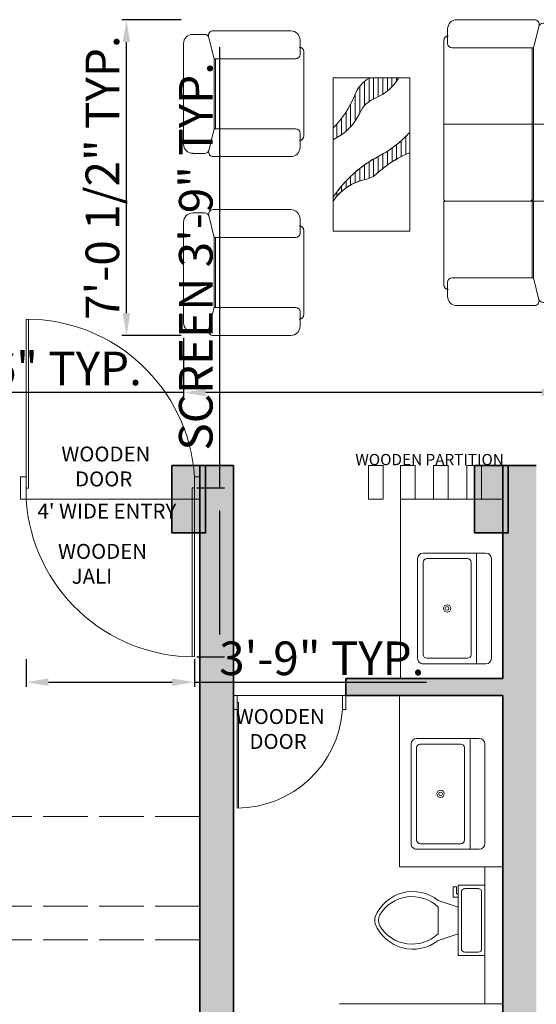
# Model space of a CAD drawing. Units: millimetres. Extents: x 595116 to 630915, y 909473 to 920225.
# Tile 130 of 134: x 630446 to 630585, y 919466 to 919729. Entities that reach past the tile are written whole.
import ezdxf

# ---------------------------------------------------------------- set-up
doc = ezdxf.new("R2010")
doc.units = ezdxf.units.MM
doc.linetypes.add('ACAD_ISO02W100', pattern=[15, 12, -3])
for name, color, linetype, lineweight in [('A-FLOR-FIXT', 9, 'Continuous', 18), ('A-FLOR-SCRN', 31, 'Continuous', 18), ('A-FLOR-SCRN-OVHD', 31, 'ACAD_ISO02W100', 13), ('A-FURN', 32, 'Continuous', 18), ('A-WALL', 1, 'Continuous', 35), ('A-WALL-PATT', 8, 'Continuous', 13), ('Column', 6, 'Continuous', 35), ('Dimension', 3, 'Continuous', 18), ('Doors', 31, 'Continuous', 20), ('Text', 7, 'Continuous', 18)]:
    doc.layers.add(name, color=color, linetype=linetype, lineweight=lineweight)
doc.styles.get("Standard").update_dxf_attribs({"font": 'arial.ttf'})
doc.dimstyles.new('ISO-25', dxfattribs={"dimtxt": 9, "dimasz": 6, "dimexe": 1.25, "dimexo": 0.625, "dimtad": 1, "dimlunit": 4, "dimtxsty": 'Standard', "dimcen": 2.5, "dimadec": 0, "dimazin": 0, "dimtfac": 1, "dimtmove": 0, "dimatfit": 3, "dimfxl": 1, "dimarcsym": 0})

# ---------------------------------------------------------------- blocks, each defined once
blk = doc.blocks.new('KWD')
for points in [[(629753.63, 919957.93), (629752.54, 919957.93), (629752.54, 919953.43), (629753.63, 919953.43)], [(629787.45, 919957.93), (629787.45, 919953.43), (629788.54, 919953.43), (629788.54, 919957.93)]]:
    blk.add_lwpolyline(points, close=True)
blk.add_lwpolyline([(629753.63, 919921.79), (629753.63, 919955.68), (629754.13, 919955.68), (629754.13, 919921.8)])
blk.add_arc((629753.64, 919955.68), 33.88, 269.99, 356.196)
blk = doc.blocks.new('DS')
blk.add_lwpolyline([(630069.78, 919993.92), (630069.78, 919965.68), (630069.37, 919965.68), (630069.37, 919993.91)])
for points in [[(630041.6, 919963.81), (630041.6, 919967.56), (630040.69, 919967.56), (630040.69, 919963.81)], [(630069.78, 919963.81), (630070.69, 919963.81), (630070.69, 919967.56), (630069.78, 919967.56)]]:
    blk.add_lwpolyline(points, close=True)
blk.add_arc((630069.78, 919965.69), 28.24, 89.99, 176.196)
blk = doc.blocks.new('Sink-single - 30 in top')
blk.add_line((-15, -3.999996), (15, -3.999996))
for points in [[(-13.5, 0), (13.5, 0)], [(-15, -18.499996), (-15, -1.5)], [(15, -1.5), (15, -18.499996)], [(-13.5, -17.499996), (-13.5, -6.499996)], [(-12.5, -5.499996), (12.5, -5.499996)], [(13.5, -6.499996), (13.5, -17.499996)], [(12.5, -18.499996), (-12.5, -18.499996)], [(13.5, -19.999996), (-13.5, -19.999996)]]:
    blk.add_lwpolyline(points)
for radius in [1, 0.5]:
    blk.add_circle((0, -11.999996), radius)
for centre, radius, start, end in [((-13.5, -1.5), 1.5, 90, 180), ((13.5, -1.5), 1.5, 0, 90), ((-12.5, -6.499996), 1, 90, 180), ((12.5, -6.499996), 1, 0, 90), ((-13.5, -18.499996), 1.5, 180, 270), ((-12.5, -17.499996), 1, 180, 270), ((12.5, -17.499996), 1, 270, 0), ((13.5, -18.499996), 1.5, 270, 0)]:
    blk.add_arc(centre, radius, start, end)
blk = doc.blocks.new('Toilet - top')
for p, q in [((9.5, -6), (9.5, -2)), ((-10, -8.5), (-8, -8.5)), ((-10, -9.5), (-10, -8.5)), ((-8, -8.5), (-8, -8)), ((-7, -8), (-7, -9.5)), ((-4, -8), (-6, -14)), ((4, -8), (6, -14)), ((-7, -9.5), (-10, -9.5)), ((4, -14), (-4, -14))]:
    blk.add_line(p, q)
blk.add_lwpolyline([(10.5, -8), (10.5, 0), (-10.5, 0), (-10.5, -8)], close=True)
for points in [[(-9.5, -2), (-9.5, -6)], [(8.5, -1), (-8.5, -1)], [(-8.5, -7), (8.5, -7)]]:
    blk.add_lwpolyline(points)
for centre, radius, start, end in [((-8.62, -1.88), 0.884, 81.8699, 188.1301), ((8.62, -1.88), 0.884, 351.8699, 98.1301), ((-8.62, -6.12), 0.884, 171.8699, 278.1301), ((8.62, -6.12), 0.884, 261.8699, 8.1301), ((3.52, -21.58), 12.17, 141.4691, 247.9714), ((4.2, -21.82), 11.33, 136.3677, 238.9468), ((-3.52, -21.58), 12.17, 292.0284, 38.5307), ((-4.2, -21.82), 11.33, 301.053, 43.6321), ((0, -27.88), 4, 245.7318, 294.2682), ((0, -29), 4, 254.8605, 285.1395)]:
    blk.add_arc(centre, radius, start, end)
blk = doc.blocks.new('SOFA')
for p, q in [((629520.59, 919742.63), (629517.45, 919742.63)), ((629517.45, 919742.63), (629520.59, 919742.63)), ((629543.7, 919743.59), (629522.89, 919743.59)), ((629522.89, 919743.59), (629543.7, 919743.59)), ((629514.98, 919740.17), (629514.98, 919695.65)), ((629514.98, 919695.65), (629514.98, 919740.17)), ((629521.79, 919741.7), (629521.7, 919742.06)), ((629521.7, 919742.06), (629523.2, 919736.06)), ((629546.16, 919741.12), (629546.16, 919739.22)), ((629546.16, 919741.12), (629546.16, 919737.29)), ((629588.11, 919740.62), (629608.91, 919740.62)), ((629588.11, 919740.62), (629608.91, 919740.62)), ((629547.17, 919738.01), (629547.17, 919695.65)), ((629547.17, 919738.01), (629547.17, 919695.65)), ((629585.64, 919738.15), (629585.64, 919734.33)), ((629585.64, 919736.25), (629585.64, 919738.15)), ((629610.11, 919739.09), (629608.61, 919733.09)), ((629610.11, 919739.09), (629610.02, 919738.73)), ((629611.21, 919739.66), (629614.36, 919739.66)), ((629611.21, 919739.66), (629614.36, 919739.66)), ((629523.2, 919736.06), (629523.2, 919695.65)), ((629523.2, 919695.65), (629523.2, 919736.06)), ((629523.2, 919695.65), (629523.2, 919736.06)), ((629544.93, 919736.06), (629523.2, 919736.06)), ((629523.2, 919736.06), (629523.53, 919736.06)), ((629523.2, 919736.06), (629523.53, 919736.06)), ((629523.53, 919736.06), (629523.53, 919695.65)), ((629523.53, 919736.06), (629523.53, 919695.65)), ((629523.53, 919736.06), (629523.53, 919695.65)), ((629584.64, 919735.04), (629584.64, 919712.53)), ((629584.64, 919712.53), (629584.64, 919735.04)), ((629616.82, 919737.2), (629616.82, 919710.3)), ((629616.82, 919737.2), (629616.82, 919710.3)), ((629586.87, 919733.09), (629608.61, 919733.09)), ((629608.28, 919733.09), (629608.61, 919733.09)), ((629608.28, 919714.4), (629608.28, 919733.09)), ((629608.28, 919733.09), (629608.28, 919714.4)), ((629608.61, 919733.09), (629608.61, 919714.4)), ((629608.61, 919733.09), (629608.61, 919714.4)), ((629556.25, 919728.06), (629556.25, 919687.01)), ((629556.25, 919687.01), (629556.25, 919728.06)), ((629576.77, 919728.06), (629556.25, 919728.06)), ((629556.25, 919728.06), (629576.77, 919728.06)), ((629559.82, 919728), (629559.82, 919727.13)), ((629561.06, 919728), (629561.06, 919725.63)), ((629562.29, 919728), (629562.29, 919724.5)), ((629563.52, 919728), (629563.52, 919723.63)), ((629564.75, 919728), (629564.75, 919722.96)), ((629565.98, 919728), (629565.98, 919722.42)), ((629567.19, 919727.97), (629567.19, 919721.68)), ((629568.42, 919727.08), (629568.42, 919720.54)), ((629576.77, 919687.01), (629576.77, 919728.06)), ((629576.77, 919728.06), (629576.77, 919687.01)), ((629569.65, 919725.8), (629569.65, 919718.67)), ((629569.65, 919725.8), (629569.65, 919718.67)), ((629570.88, 919723.75), (629570.88, 919716.49)), ((629570.88, 919716.49), (629570.88, 919723.75)), ((629572.12, 919720.99), (629572.12, 919714.94)), ((629573.35, 919718.86), (629573.35, 919713.74)), ((629574.58, 919717.12), (629574.58, 919712.78)), ((629547.17, 919715.59), (629514.98, 919715.59)), ((629575.81, 919715.64), (629575.81, 919712.02)), ((629586.87, 919714.4), (629608.61, 919714.4)), ((629608.61, 919714.4), (629608.28, 919714.4)), ((629610.09, 919708.48), (629608.61, 919714.4)), ((629557.33, 919712.4), (629557.33, 919707.56)), ((629557.33, 919707.56), (629557.33, 919712.4)), ((629558.57, 919711.23), (629558.57, 919706.97)), ((629585.64, 919709.42), (629585.64, 919713.17)), ((629585.64, 919709.42), (629585.64, 919711.32)), ((629559.8, 919710.18), (629559.8, 919706.31)), ((629561.03, 919709.25), (629561.03, 919705.57)), ((629562.26, 919708.41), (629562.26, 919704.73)), ((629610.02, 919708.77), (629610.09, 919708.48)), ((629563.49, 919707.66), (629563.49, 919703.8)), ((629564.72, 919706.99), (629564.72, 919702.74)), ((629565.96, 919706.31), (629565.96, 919701.75)), ((629588.11, 919706.95), (629608.89, 919706.95)), ((629608.89, 919706.95), (629588.11, 919706.95)), ((629611.21, 919707.83), (629611.48, 919707.83)), ((629611.48, 919707.83), (629611.21, 919707.83)), ((629611.48, 919707.83), (629614.36, 919707.83)), ((629614.36, 919707.83), (629611.48, 919707.83)), ((629567.19, 919705.56), (629567.19, 919701.12)), ((629568.42, 919704.73), (629568.42, 919700.78)), ((629569.65, 919703.81), (629569.65, 919700.45)), ((629570.88, 919702.8), (629570.88, 919699.98)), ((629572.12, 919701.68), (629572.12, 919699.37)), ((629573.35, 919700.43), (629573.35, 919698.59)), ((629574.58, 919699.04), (629574.58, 919697.6)), ((629575.81, 919697.48), (629575.81, 919696.34)), ((629575.81, 919697.48), (629575.81, 919696.34)), ((629547.17, 919695.06), (629514.98, 919695.06)), ((629514.98, 919695.06), (629514.98, 919670.42)), ((629514.98, 919670.42), (629514.98, 919695.06)), ((629514.98, 919695.06), (629515.44, 919695.06)), ((629515.6, 919695.04), (629546.55, 919695.04)), ((629523.2, 919695.06), (629523.2, 919674.53)), ((629523.2, 919674.53), (629523.2, 919695.04)), ((629523.2, 919674.53), (629523.2, 919695.04)), ((629523.2, 919695.04), (629523.53, 919695.04)), ((629523.2, 919695.04), (629523.53, 919695.04)), ((629523.53, 919695.04), (629523.53, 919695.11)), ((629523.53, 919695.04), (629523.53, 919695.11)), ((629523.53, 919695.06), (629523.53, 919674.53)), ((629523.53, 919695.04), (629523.53, 919674.53)), ((629523.53, 919695.04), (629523.53, 919674.53)), ((629524.14, 919695.04), (629523.53, 919695.04)), ((629524.14, 919695.04), (629523.53, 919695.04)), ((629546.71, 919695.06), (629547.17, 919695.06)), ((629547.17, 919695.06), (629547.17, 919672.66)), ((629547.17, 919695.06), (629547.17, 919672.66)), ((629588.11, 919692.76), (629608.89, 919692.76)), ((629608.89, 919692.76), (629588.11, 919692.76)), ((629585.64, 919690.3), (629585.64, 919688.39)), ((629585.64, 919690.3), (629585.64, 919686.55)), ((629610.09, 919691.23), (629608.61, 919685.31)), ((629610.02, 919690.95), (629610.09, 919691.23)), ((629611.21, 919691.88), (629611.48, 919691.88)), ((629611.48, 919691.88), (629611.21, 919691.88)), ((629611.48, 919691.88), (629614.36, 919691.88)), ((629614.36, 919691.88), (629611.48, 919691.88)), ((629616.82, 919662.52), (629616.82, 919689.42)), ((629616.82, 919662.52), (629616.82, 919689.42)), ((629556.25, 919687.01), (629576.77, 919687.01)), ((629576.77, 919687.01), (629556.25, 919687.01)), ((629584.64, 919664.68), (629584.64, 919687.18)), ((629584.64, 919687.18), (629584.64, 919664.68)), ((629586.87, 919685.31), (629608.61, 919685.31)), ((629608.61, 919685.31), (629608.28, 919685.31)), ((629608.28, 919685.31), (629608.28, 919666.62)), ((629608.28, 919666.62), (629608.28, 919685.31)), ((629608.61, 919666.62), (629608.61, 919685.31)), ((629608.61, 919666.62), (629608.61, 919685.31)), ((629521.72, 919668.61), (629523.2, 919674.53)), ((629544.93, 919674.53), (629523.2, 919674.53)), ((629523.53, 919674.53), (629523.2, 919674.53)), ((629523.53, 919674.53), (629523.2, 919674.53)), ((629546.16, 919669.54), (629546.16, 919673.3)), ((629521.72, 919668.61), (629521.79, 919668.89)), ((629546.16, 919671.45), (629546.16, 919669.54)), ((629520.32, 919667.96), (629517.45, 919667.96)), ((629520.32, 919667.96), (629517.45, 919667.96)), ((629520.59, 919667.96), (629520.32, 919667.96)), ((629520.59, 919667.96), (629520.32, 919667.96)), ((629543.7, 919667.08), (629522.91, 919667.08)), ((629543.7, 919667.08), (629522.91, 919667.08)), ((629586.87, 919666.62), (629608.61, 919666.62)), ((629608.28, 919666.62), (629608.61, 919666.62)), ((629610.11, 919660.63), (629608.61, 919666.62)), ((629585.64, 919661.56), (629585.64, 919665.39)), ((629585.64, 919663.47), (629585.64, 919661.56)), ((629610.11, 919660.63), (629610.02, 919660.99)), ((629588.11, 919659.1), (629608.91, 919659.1)), ((629588.11, 919659.1), (629608.91, 919659.1)), ((629611.21, 919660.05), (629614.36, 919660.05)), ((629611.21, 919660.05), (629614.36, 919660.05))]:
    blk.add_line(p, q)
for centre, radius, start, end in [((629517.45, 919740.17), 2.46, 90, 180), ((629517.45, 919740.17), 2.46, 90, 180), ((629520.59, 919741.4), 1.23, 14.0362, 90), ((629520.59, 919741.4), 1.23, 14.0362, 90), ((629522.89, 919742.36), 1.23, 90, 194.0362), ((629522.89, 919742.36), 1.23, 90, 194.0362), ((629543.7, 919741.12), 2.46, 0, 90), ((629543.7, 919741.12), 2.46, 0, 90), ((629588.11, 919738.15), 2.46, 90, 180), ((629588.11, 919738.15), 2.46, 90, 180), ((629608.91, 919739.39), 1.23, 345.9638, 90), ((629608.91, 919739.39), 1.23, 345.9638, 90), ((629545.94, 919738.01), 1.23, 0, 90), ((629545.94, 919738.01), 1.23, 0, 79.4007), ((629611.21, 919738.43), 1.23, 90, 165.9638), ((629611.21, 919738.43), 1.23, 90, 165.9638), ((629614.36, 919737.2), 2.46, 0, 90), ((629614.36, 919737.2), 2.46, 0, 90), ((629544.93, 919737.29), 1.23, 270, 0), ((629585.87, 919735.04), 1.23, 90, 180), ((629585.87, 919735.04), 1.23, 100.5993, 180), ((629586.87, 919734.33), 1.23, 180, 270), ((629570.11, 919734.3), 12.54, 210.2644, 248.0021), ((629562.37, 919720.03), 9.29, 21.2599, 58.8091), ((629562.37, 919720.03), 9.29, 23.6102, 38.4008), ((629562.42, 919715.26), 7.99, 24.8088, 68.0021), ((629594.57, 919732.56), 25.26, 201.2599, 225.1217), ((629582.84, 919724.7), 14.51, 204.5645, 214.4539), ((629582.84, 919724.7), 14.51, 204.8088, 245.1378), ((629586.87, 919713.17), 1.23, 90, 180), ((629577.93, 919732.79), 28.98, 222.2366, 242.5747), ((629577.93, 919732.79), 28.98, 224.7026, 242.5747), ((629585.87, 919712.53), 1.23, 180, 270), ((629585.87, 919712.53), 1.23, 180, 259.4007), ((629588.11, 919709.42), 2.46, 180, 270), ((629588.11, 919709.42), 2.46, 180, 270), ((629608.89, 919708.18), 1.23, 270, 14.0362), ((629608.89, 919708.18), 1.23, 270, 14.0362), ((629611.21, 919709.06), 1.23, 194.0362, 270), ((629611.21, 919709.06), 1.23, 194.0362, 270), ((629614.36, 919710.3), 2.46, 270, 0), ((629614.36, 919710.3), 2.46, 270, 0), ((629546.11, 919682.25), 27.68, 46.9747, 68.4773), ((629546.11, 919682.25), 27.68, 46.9747, 66.0851), ((629549.56, 919678.1), 32.63, 33.5604, 62.5747), ((629549.56, 919678.1), 32.63, 36.4252, 62.5747), ((629569.57, 919707.39), 6.7, 226.9747, 258.3827), ((629569.57, 919707.39), 6.7, 226.9746, 258.3828), ((629565.49, 919687.55), 13.55, 33.8658, 78.3827), ((629565.49, 919687.55), 13.55, 40.4201, 78.3827), ((629515.6, 919695.65), 0.616, 180, 270), ((629515.6, 919695.65), 0.616, 180, 255.079), ((629523.81, 919695.65), 0.616, 180, 270), ((629523.81, 919695.65), 0.616, 180, 242.2854), ((629523.81, 919695.65), 0.616, 180, 242.2854), ((629524.14, 919695.65), 0.616, 180, 270), ((629524.14, 919695.65), 0.616, 180, 270), ((629524.14, 919695.65), 0.616, 180, 270), ((629546.55, 919695.65), 0.616, 270, 0), ((629546.55, 919695.65), 0.616, 284.921, 0), ((629588.11, 919690.3), 2.46, 90, 180), ((629588.11, 919690.3), 2.46, 90, 180), ((629608.89, 919691.53), 1.23, 345.9638, 90), ((629608.89, 919691.53), 1.23, 345.9638, 90), ((629611.21, 919690.65), 1.23, 90, 165.9638), ((629611.21, 919690.65), 1.23, 90, 165.9638), ((629614.36, 919689.42), 2.46, 0, 90), ((629614.36, 919689.42), 2.46, 0, 90), ((629585.87, 919687.18), 1.23, 90, 180), ((629585.87, 919687.18), 1.23, 100.5993, 180), ((629586.87, 919686.55), 1.23, 180, 270), ((629544.93, 919673.3), 1.23, 0, 90), ((629545.94, 919672.66), 1.23, 270, 0), ((629545.94, 919672.66), 1.23, 280.5993, 0), ((629517.45, 919670.42), 2.46, 180, 270), ((629517.45, 919670.42), 2.46, 180, 270), ((629520.59, 919669.19), 1.23, 270, 345.9638), ((629520.59, 919669.19), 1.23, 270, 345.9638), ((629543.7, 919669.54), 2.46, 270, 0), ((629543.7, 919669.54), 2.46, 270, 0), ((629522.91, 919668.31), 1.23, 165.9638, 270), ((629522.91, 919668.31), 1.23, 165.9638, 270), ((629586.87, 919665.39), 1.23, 90, 180), ((629585.87, 919664.68), 1.23, 180, 270), ((629585.87, 919664.68), 1.23, 180, 259.4007), ((629588.11, 919661.56), 2.46, 180, 270), ((629588.11, 919661.56), 2.46, 180, 270), ((629611.21, 919661.28), 1.23, 194.0362, 270), ((629611.21, 919661.28), 1.23, 194.0362, 270), ((629614.36, 919662.52), 2.46, 270, 0), ((629614.36, 919662.52), 2.46, 270, 0), ((629608.91, 919660.33), 1.23, 270, 14.0362), ((629608.91, 919660.33), 1.23, 270, 14.0362)]:
    blk.add_arc(centre, radius, start, end)
at = {"flags": 9}
for tag in ['XSIZE', 'YSIZE']:
    blk.add_attdef(tag, (629556.25, 919728.06), '', height=0.0205, rotation=270, dxfattribs=at)
blk = doc.blocks.new('DOOR-ENTRY-SCREEN')
blk.add_lwpolyline([(45.09, 0), (45.09, 45.18), (44.42, 45.18), (44.42, 0.01)])
blk.add_arc((45.08, 45.18), 45.18, 183.804, 270.01)
blk = doc.blocks.new('COLUMN-RECT-9X18')
h = blk.add_hatch(color=256)
h.dxf.hatch_style = 1
h.paths.add_polyline_path([(9, 18), (0, 18), (0, 0), (9, 0)])
blk.add_lwpolyline([(0, 18), (9, 18), (9, 0), (0, 0)], close=True)
blk = doc.blocks.new('*D182')
at = {"layer": 'Defpoints', "color": 0, "transparency": 16777216}
for p in [(630490.2, 919644.73), (630592.04, 919644.73), (630490.2, 919629.46)]:
    blk.add_point(p, dxfattribs=at)
at = {"layer": 'Dimension', "color": 0, "lineweight": -2, "transparency": 16777216}
for p, q in [((630490.2, 919644.11), (630490.2, 919628.21)), ((630592.04, 919644.11), (630592.04, 919628.21)), ((630490.2, 919629.46), (630340.81, 919629.46)), ((630586.04, 919629.46), (630496.2, 919629.46))]:
    blk.add_line(p, q, dxfattribs=at)
at = {"layer": 'Dimension', "color": 0, "transparency": 16777216}
for points in [[(630496.2, 919630.46), (630496.2, 919628.46), (630490.2, 919629.46)], [(630586.04, 919630.46), (630586.04, 919628.46), (630592.04, 919629.46)]]:
    blk.add_solid(points, dxfattribs=at)
at = {"layer": 'Dimension', "color": 0, "transparency": 16777216, "insert": (630412.5, 919634.74), "char_height": 9, "attachment_point": 5}
blk.add_mtext('SOFA GROUP 8\'-6" TYP.', dxfattribs=at)
blk = doc.blocks.new('*D183')
at = {"layer": 'Defpoints', "color": 0, "transparency": 16777216}
for p in [(630474.92, 919729.22), (630490.2, 919729.22), (630490.2, 919644.73)]:
    blk.add_point(p, dxfattribs=at)
at = {"layer": 'Dimension', "color": 0, "lineweight": -2, "transparency": 16777216}
for p, q in [((630489.57, 919729.22), (630473.67, 919729.22)), ((630474.92, 919650.73), (630474.92, 919723.22)), ((630489.57, 919644.73), (630473.67, 919644.73))]:
    blk.add_line(p, q, dxfattribs=at)
at = {"layer": 'Dimension', "color": 0, "transparency": 16777216}
for points in [[(630473.92, 919723.22), (630475.92, 919723.22), (630474.92, 919729.22)], [(630473.92, 919650.73), (630475.92, 919650.73), (630474.92, 919644.73)]]:
    blk.add_solid(points, dxfattribs=at)
at = {"layer": 'Dimension', "color": 0, "transparency": 16777216, "insert": (630469.64, 919686.98), "char_height": 9, "attachment_point": 5, "rotation": 90}
blk.add_mtext('7\'-0 1/2" TYP.', dxfattribs=at)
blk = doc.blocks.new('*D198')
at = {"layer": 'Defpoints', "color": 0, "transparency": 16777216}
for p in [(630493.14, 919603.93), (630499.92, 919603.93), (630493.14, 919558.74)]:
    blk.add_point(p, dxfattribs=at)
at = {"layer": 'Dimension', "color": 0, "lineweight": -2, "transparency": 16777216}
for p, q in [((630499.92, 919603.93), (630499.92, 919721.88)), ((630493.76, 919603.93), (630501.17, 919603.93)), ((630499.92, 919564.74), (630499.92, 919597.93)), ((630493.76, 919558.74), (630501.17, 919558.74))]:
    blk.add_line(p, q, dxfattribs=at)
at = {"layer": 'Dimension', "color": 0, "transparency": 16777216}
for points in [[(630498.92, 919597.93), (630500.92, 919597.93), (630499.92, 919603.93)], [(630498.92, 919564.74), (630500.92, 919564.74), (630499.92, 919558.74)]]:
    blk.add_solid(points, dxfattribs=at)
at = {"layer": 'Dimension', "color": 0, "transparency": 16777216, "insert": (630494.63, 919665.91), "char_height": 9, "attachment_point": 5, "rotation": 90}
blk.add_mtext('SCREEN 3\'-9" TYP.', dxfattribs=at)
blk = doc.blocks.new('*D199')
at = {"layer": 'Defpoints', "color": 0, "transparency": 16777216}
for p in [(630448.05, 919558.74), (630493.14, 919558.74), (630493.14, 919551.97)]:
    blk.add_point(p, dxfattribs=at)
at = {"layer": 'Dimension', "color": 0, "lineweight": -2, "transparency": 16777216}
for p, q in [((630448.05, 919558.12), (630448.05, 919550.72)), ((630493.14, 919558.12), (630493.14, 919550.72)), ((630454.05, 919551.97), (630487.14, 919551.97)), ((630493.14, 919551.97), (630555.24, 919551.97))]:
    blk.add_line(p, q, dxfattribs=at)
at = {"layer": 'Dimension', "color": 0, "transparency": 16777216}
for points in [[(630454.05, 919552.97), (630454.05, 919550.97), (630448.05, 919551.97)], [(630487.14, 919552.97), (630487.14, 919550.97), (630493.14, 919551.97)]]:
    blk.add_solid(points, dxfattribs=at)
at = {"layer": 'Dimension', "color": 0, "transparency": 16777216, "insert": (630527.19, 919557.19), "char_height": 9, "attachment_point": 5}
blk.add_mtext('3\'-9" TYP.', dxfattribs=at)

msp = doc.modelspace()

# ---------------------------------------------------------------- hatches: boundary and pattern name
at = {"layer": 'A-WALL-PATT'}
h = msp.add_hatch(color=256, dxfattribs=at)
h.dxf.hatch_style = 1
h.paths.add_polyline_path([(630503.596, 919609.928), (630496.096, 919609.928), (630496.096, 919591.928), (630494.596, 919591.928), (630494.596, 919429.828), (630496.096, 919429.828), (630496.096, 919411.928), (630512.596, 919411.928), (630512.596, 919420.323), (630536.596, 919420.323), (630536.596, 919411.928), (630575.596, 919411.928), (630575.596, 919420.928), (630503.596, 919420.928)])
h = msp.add_hatch(color=256, dxfattribs=at)
h.dxf.hatch_style = 1
h.paths.add_polyline_path([(630584.596, 919609.928), (630577.096, 919609.928), (630577.096, 919591.928), (630575.596, 919591.928), (630575.596, 919552.928), (630533.596, 919552.928), (630533.596, 919548.428), (630575.596, 919548.428), (630575.596, 919429.928), (630577.096, 919429.928), (630577.096, 919411.928), (630608.596, 919411.928), (630608.596, 919420.928), (630584.596, 919420.928)])

# ---------------------------------------------------------------- linework, layer by layer
at = {"layer": 'A-FLOR-FIXT'}
for p, q in [((630575.596, 919600.928), (630548.211, 919600.928)), ((630548.211, 919600.928), (630548.211, 919552.928)), ((630547.996, 919548.428), (630547.996, 919502.538)), ((630547.996, 919502.538), (630575.596, 919502.538)), ((630570.826, 919502.538), (630570.826, 919465.872)), ((630575.596, 919465.872), (630531.887, 919465.872))]:
    msp.add_line(p, q, dxfattribs=at)
at = {"layer": 'A-FLOR-SCRN'}
for points in [[(630543.597, 919600.928), (630539.649, 919600.928), (630539.649, 919609.928), (630543.597, 919609.928)], [(630552.16, 919600.928), (630548.211, 919600.928), (630548.211, 919609.928), (630552.16, 919609.928)], [(630561.044, 919600.928), (630557.095, 919600.928), (630557.095, 919609.928), (630561.044, 919609.928)], [(630569.951, 919600.928), (630566.003, 919600.928), (630566.003, 919609.928), (630569.951, 919609.928)]]:
    msp.add_lwpolyline(points, close=True, dxfattribs=at)
at = {"layer": 'A-FLOR-SCRN-OVHD'}
for p, q in [((630302.596, 919516.015), (630494.596, 919516.015)), ((630302.596, 919492.015), (630494.596, 919492.015)), ((630302.596, 919483.015), (630494.596, 919483.015))]:
    msp.add_line(p, q, dxfattribs=at)
at = {"layer": 'A-WALL'}
for p, q in [((630494.596, 919411.928), (630494.596, 919609.928)), ((630494.596, 919609.928), (630503.596, 919609.928)), ((630503.596, 919420.928), (630503.596, 919609.928)), ((630575.596, 919552.928), (630575.596, 919609.928)), ((630575.596, 919609.928), (630584.596, 919609.928)), ((630533.596, 919548.428), (630533.596, 919552.928)), ((630533.596, 919552.928), (630575.596, 919552.928)), ((630533.596, 919548.428), (630575.596, 919548.428)), ((630575.596, 919420.928), (630575.596, 919548.428))]:
    msp.add_line(p, q, dxfattribs=at)
at = {"layer": 'Doors'}
for p, q in [((630487.096, 919609.928), (630496.096, 919609.928)), ((630448.053, 919600.928), (630493.139, 919600.928)), ((630532.685, 919548.428), (630504.507, 919548.428))]:
    msp.add_line(p, q, dxfattribs=at)

# ---------------------------------------------------------------- block references
at = {"layer": 'A-FLOR-FIXT', "rotation": 270}
for name, p, xscale, yscale, zscale in [('Sink-single - 30 in top', (630572.577, 919571.697), 0.9872623020467125, 0.9872623020467125, 0.9872623020467125), ('Sink-single - 30 in top', (630570.825, 919522.087), 0.9872623020467125, 0.9872623020467125, 0.9872623020467125), ('Toilet - top', (630570.826, 919488.247), 0.8924547258250047, 0.8924547258250047, 0.8924547258250047)]:
    msp.add_blockref(name, p, dxfattribs=dict(at, xscale=xscale, yscale=yscale, zscale=zscale))
at = {"layer": 'A-FURN', "xscale": -1}
msp.add_blockref('SOFA', (1260107.02, -14.364), dxfattribs=at)
at = {"layer": 'Column'}
for p in [(630487.096, 919591.928), (630568.096, 919591.928)]:
    msp.add_blockref('COLUMN-RECT-9X18', p, dxfattribs=at)
at = {"layer": 'Doors', "xscale": -1.333333333333333, "yscale": 1.333333333333333, "zscale": 1.333333333333333, "rotation": 180}
msp.add_blockref('KWD', (-209223.458, 2146211.498), dxfattribs=at)
at = {"layer": 'Doors'}
msp.add_blockref('DOOR-ENTRY-SCREEN', (630448.053, 919558.748), dxfattribs=at)
at = {"layer": 'Doors', "rotation": 180}
msp.add_blockref('DS', (1260574.29, 1839512.237), dxfattribs=at)

# ---------------------------------------------------------------- texts
at = {"layer": 'Text', "attachment_point": 1}
for s, insert, char_height in [('{     WOODEN\\P        DOOR}', (630451.388, 919615.018), 4), ('{ WOODEN PARTITION}', (630535.258, 919613.032), 3), ("{4' WIDE ENTRY}", (630451.109, 919599.749), 4), ('{     WOODEN\\P        JALI}', (630450.501, 919588.969), 4), ('{     WOODEN\\P        DOOR}', (630498.055, 919544.782), 4)]:
    msp.add_mtext_dynamic_manual_height_columns(s, width=61.33456, gutter_width=12.5, heights=[0], dxfattribs=dict(at, insert=insert, char_height=char_height))

# ---------------------------------------------------------------- dimensions: what is measured, and where the dimension line sits
at = {"layer": 'Dimension'}
for base, p1, p2, angle, text, picture, middle in [((630474.923, 919729.223), (630490.198, 919644.733), (630490.198, 919729.223), 90, '<> TYP.', '*D183', (630469.644, 919686.978)), ((630499.916, 919603.928), (630493.139, 919558.743), (630493.139, 919603.928), 90, 'SCREEN <> TYP.', '*D198', (630494.635, 919665.906)), ((630490.198, 919629.458), (630592.035, 919644.733), (630490.198, 919644.733), 180, 'SOFA GROUP <> TYP.', '*D182', (630412.503, 919634.739))]:
    dim = msp.add_linear_dim(base=base, p1=p1, p2=p2, angle=angle, text=text, dimstyle='ISO-25', override={"dimdec": 1, "dimlfac": 1, "dimrnd": 0, "dimzin": 1, "dimdsep": 46, "dimlunit": 4, "dimfrac": 2}, dxfattribs=at)
    dim.commit()
    dim.dimension.update_dxf_attribs({"geometry": picture, "text_midpoint": middle})
dim = msp.add_linear_dim(base=(630493.139, 919551.966), p1=(630448.053, 919558.743), p2=(630493.139, 919558.743), text='<> TYP.', dimstyle='ISO-25', override={"dimdec": 1, "dimlfac": 1, "dimrnd": 0, "dimzin": 1, "dimdsep": 46, "dimlunit": 4, "dimfrac": 2}, dxfattribs=at)
dim.commit()
dim.dimension.update_dxf_attribs({"geometry": '*D199', "text_midpoint": (630527.19, 919557.189)})

doc.saveas('drawing.dxf')
